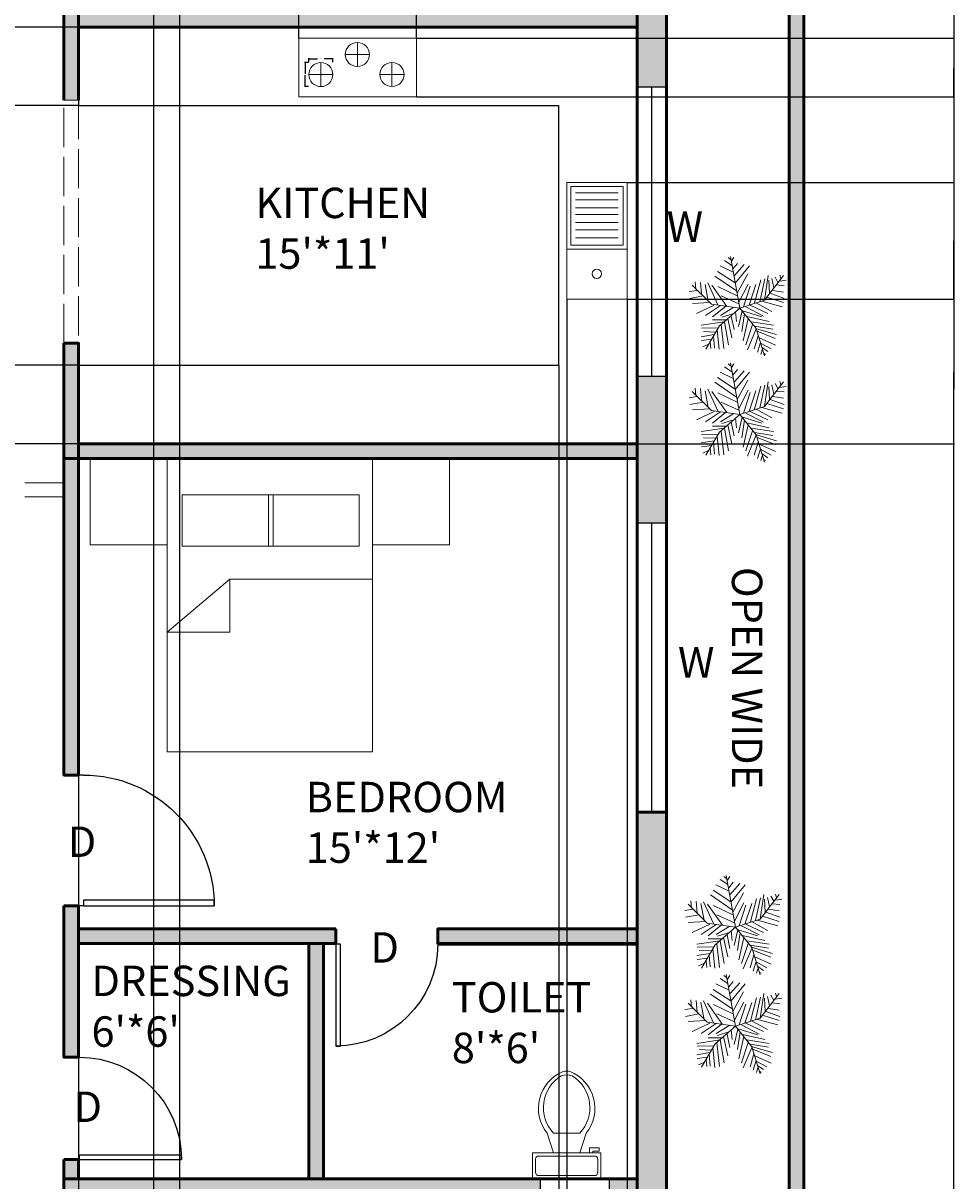
# Model space of a CAD drawing. Units: inches. Extents: x 2024 to 2594, y 643 to 1604.
# Tile 3 of 4: x 2309 to 2594, y 865 to 1219. Entities that reach past the tile are written whole.
import ezdxf

# ---------------------------------------------------------------- set-up
doc = ezdxf.new("R2010")
doc.units = ezdxf.units.IN
doc.linetypes.add('ACAD_ISO02W100', pattern=[15, 12, -3])
for name, color, linetype, lineweight in [('A-ANNO-DIMS', 2, 'Continuous', 18), ('A-ANNO-TEXT', 7, 'Continuous', 18), ('A-AREA-IDEN', 7, 'Continuous', 25), ('A-EQPM', 8, 'Continuous', 18), ('A-FLOR-CASE', 30, 'Continuous', 25), ('A-FLOR-FIXT', 8, 'Continuous', 18), ('A-WALL-OVHD', 50, 'ACAD_ISO02W100', 18), ('A-WALL-PATT', 50, 'Continuous', 13), ('C-PROP', 7, 'Continuous', 35), ('DOOR', 240, 'Continuous', 25), ('FUR', 212, 'Continuous', 18), ('TREE', 102, 'Continuous', 18), ('WALL', 50, 'Continuous', 50), ('WIN', 140, 'Continuous', 25)]:
    doc.layers.add(name, color=color, linetype=linetype, lineweight=lineweight)
doc.styles.get("Standard").update_dxf_attribs({"font": 'arial.ttf'})
doc.dimstyles.get("Standard").update_dxf_attribs({"dimtxt": 0.18, "dimasz": 0.18, "dimexe": 0.18, "dimexo": 0.0625, "dimgap": 0.09, "dimtad": 0, "dimtih": 1, "dimtoh": 1, "dimdec": 4, "dimzin": 0, "dimdsep": 46, "dimtxsty": 'Standard', "dimcen": 0.09, "dimadec": 0, "dimazin": 0, "dimtfac": 1, "dimtdec": 4, "dimtofl": 0, "dimtmove": 0, "dimatfit": 3, "dimfxl": 1, "dimtolj": 1, "dimtzin": 0, "dimarcsym": 0})

# ---------------------------------------------------------------- blocks, each defined once
blk = doc.blocks.new('*U4')
for p, q in [((9.5, -6), (9.5, -2)), ((-10, -8.5), (-8, -8.5)), ((-10, -9.5), (-10, -8.5)), ((-7, -9.5), (-10, -9.5)), ((-8, -8.5), (-8, -8)), ((-7, -8), (-7, -9.5)), ((-4, -8), (-6, -14)), ((4, -8), (6, -14)), ((4, -14), (-4, -14))]:
    blk.add_line(p, q)
blk.add_lwpolyline([(10.5, -8), (10.5, 0), (-10.5, 0), (-10.5, -8)], close=True)
for points in [[(-9.5, -2), (-9.5, -6)], [(8.5, -1), (-8.5, -1)], [(-8.5, -7), (8.5, -7)]]:
    blk.add_lwpolyline(points)
for centre, radius, start, end in [((-8.62, -1.88), 0.884, 81.8699, 188.1301), ((8.62, -1.88), 0.884, 351.8699, 98.1301), ((-8.62, -6.12), 0.884, 171.8699, 278.1301), ((8.62, -6.12), 0.884, 261.8699, 8.1301), ((3.52, -21.58), 12.17, 141.4691, 247.9714), ((4.2, -21.82), 11.33, 136.3677, 238.9468), ((-3.52, -21.58), 12.17, 292.0284, 38.5307), ((-4.2, -21.82), 11.33, 301.053, 43.6321), ((0, -27.88), 4, 245.7318, 294.2682), ((0, -29), 4, 254.8605, 285.1395)]:
    blk.add_arc(centre, radius, start, end)
blk = doc.blocks.new('*U2')
for p, q in [((0, 0), (0, -6)), ((40, 0), (40, -6))]:
    blk.add_line(p, q)
blk.add_lwpolyline([(0, 0), (0, 40), (1.75, 40), (1.75, 0)], close=True)
blk.add_arc((0, 0), 40, 0, 90)
blk = doc.blocks.new('*U6')
for p, q in [((-8.737, 47.138), (-17.069, 52.711)), ((-10.186, 53.64), (-13.084, 55.962)), ((0, 0), (-10.5, 57)), ((-9.099, 51.782), (-6.563, 55.962)), ((-5.114, 28.097), (-24.676, 40.636)), ((-7.288, 39.707), (-21.778, 46.673)), ((-7.65, 43.423), (-2.578, 49.46)), ((-5.839, 35.992), (4.667, 48.067)), ((-5.114, 27.632), (10.463, 46.673)), ((-48.585, 21.131), (-49.309, 29.026)), ((-43.513, 28.561), (-42.427, 15.558)), ((-38.442, 26.239), (-34.819, 7.663)), ((-35.544, 28.097), (-24.314, 3.947)), ((-3.665, 19.273), (-27.574, 35.527)), ((-2.941, 16.486), (8.652, 37.85)), ((-1.129, 6.734), (9.014, 26.704)), ((10.101, 3.483), (17.708, 26.239)), ((16.259, 5.805), (23.142, 31.348)), ((22.055, 7.198), (27.489, 32.277)), ((27, 9), (48, 36)), ((27.127, 9.056), (31.112, 35.992)), ((31.836, 30.883), (32.561, 16.486)), ((35.096, 32.741), (37.27, 22.524)), ((38.719, 34.134), (41.979, 28.561)), ((40.53, 25.775), (48.862, 24.846)), ((43.791, 29.954), (51.036, 30.883)), ((44.153, 36.456), (45.239, 32.741)), ((-47.498, 19.737), (-55.83, 18.344)), ((-40.615, 13.7), (-55.105, 10.913)), ((-31.5, 4.5), (-52.5, 25.5)), ((-14.533, 2.09), (-30.834, 25.31)), ((-24.314, 23.917), (-2.941, 13.7)), ((-20.691, 13.7), (-1.129, 4.876)), ((3.942, 1.625), (11.187, 24.381)), ((33.285, 16.486), (48.862, 10.913)), ((36.183, 19.737), (48.137, 17.88)), ((-33.37, 6.269), (-52.207, 5.34)), ((-28.299, 3.483), (-47.86, -5.805)), ((-21.416, 3.018), (-38.079, -8.128)), ((0, 0), (-31.5, 4.5)), ((-15.982, 2.09), (-30.11, -9.521)), ((0, 0), (-22.5, -19.5)), ((-6.563, 1.161), (-21.416, -8.128)), ((0, 0), (27, 9)), ((0, 0), (18, -22.5)), ((6.478, 1.625), (26.04, -8.592)), ((11.187, 3.483), (30.749, -5.805)), ((18.07, 5.805), (35.096, -3.483)), ((24.229, 7.663), (46.688, 1.625)), ((29.662, 12.307), (48.137, 6.269)), ((-6.563, -5.805), (-19.967, -9.985)), ((-13.446, -11.378), (-8.737, -32.741)), ((-9.461, -8.592), (-6.201, -23.453)), ((-4.752, -3.483), (-3.665, -14.629)), ((2.493, -3.019), (-1.491, -20.202)), ((1.769, -2.555), (24.229, -9.521)), ((5.029, -6.27), (2.131, -25.775)), ((9.014, -11.378), (3.58, -35.992)), ((7.565, -9.056), (32.198, -14.629)), ((-17.431, -15.094), (-42.789, -18.809)), ((-24.314, -21.596), (-42.427, -22.06)), ((-22.5, -19.5), (-37.5, -45)), ((-15.257, -12.772), (-30.11, -12.772)), ((-25.038, -23.918), (-22.865, -45.281)), ((-20.691, -18.345), (-17.793, -44.352)), ((-17.069, -15.094), (-12.721, -40.172)), ((14.085, -16.951), (6.478, -40.172)), ((18.07, -22.524), (8.289, -45.745)), ((12.274, -15.094), (36.907, -18.809)), ((16.259, -19.738), (36.183, -22.989)), ((18, -22.5), (27, -52.5)), ((18.433, -22.524), (40.53, -29.026)), ((19.157, -25.311), (38.719, -33.206)), ((-28.299, -29.026), (-42.789, -31.348)), ((-30.834, -34.135), (-42.427, -35.528)), ((-26.849, -26.24), (-40.253, -25.775)), ((-32.646, -36.921), (-31.921, -44.352)), ((-29.023, -30.884), (-27.936, -43.887)), ((20.244, -30.419), (15.897, -44.816)), ((22.78, -37.85), (19.519, -48.532)), ((21.331, -32.741), (39.081, -40.636)), ((-34.457, -39.708), (-40.978, -42.494)), ((22.78, -38.314), (34.372, -44.816)), ((24.591, -45.745), (23.142, -50.854)), ((24.591, -43.423), (30.749, -47.603)), ((26.764, -49.925), (28.213, -50.854))]:
    blk.add_line(p, q)
blk = doc.blocks.new('BED-DOUBLE-WITH-NIGHTSTANDS')
for p, q in [((36.91, 86.39), (36.91, 42.72)), ((36.91, 42.72), (53.2, 42.72)), ((53.2, 23.62), (36.91, 42.72)), ((53.2, 42.72), (53.2, 23.62))]:
    blk.add_line(p, q)
for points in [[(0, 86.39), (26.45, 86.39), (26.45, 110.01), (0, 110.01)], [(0, 23.62), (89.75, 23.62), (89.75, 86.39), (0, 86.39)], [(11.14, 54.55), (26.84, 54.55), (26.84, 82.37), (11.14, 82.37)], [(11.14, 28.22), (26.84, 28.22), (26.84, 56.03), (11.14, 56.03)], [(0, 0), (26.45, 0), (26.45, 23.62), (0, 23.62)]]:
    blk.add_lwpolyline(points, close=True)
blk = doc.blocks.new('COOKTOP-BURNER')
for p, q in [((3.69, 0), (3.69, 7.39)), ((0, 3.69), (7.39, 3.69))]:
    blk.add_line(p, q)
blk.add_circle((3.69, 3.69), 3.69)
blk = doc.blocks.new('WINDOW-EXTERIOR')
blk.add_line((4.5, 0), (4.5, 88.37))
blk.add_lwpolyline([(0, 0), (9, 0), (9, 88.37), (0, 88.37)], close=True)
blk = doc.blocks.new('*D21')
at = {"layer": 'A-ANNO-DIMS', "color": 0, "lineweight": -2, "transparency": 16777216}
for p, q in [((2396.73, 1207.18), (2396.73, 1208.4)), ((2396.91, 1208.22), (2399.4, 1208.22)), ((2403.94, 1208.22), (2401.44, 1208.22)), ((2404.12, 1207.18), (2404.12, 1208.4))]:
    blk.add_line(p, q, dxfattribs=at)
at = {"layer": 'A-ANNO-DIMS', "color": 0, "lineweight": 100, "transparency": 16777216}
for points in [[(2396.91, 1208.25), (2396.91, 1208.19), (2396.73, 1208.22)], [(2403.94, 1208.25), (2403.94, 1208.19), (2404.12, 1208.22)]]:
    blk.add_solid(points, dxfattribs=at)
at = {"layer": 'Defpoints', "color": 0, "lineweight": 100, "transparency": 16777216}
for p in [(2404.12, 1208.22), (2396.73, 1207.11), (2404.12, 1207.11)]:
    blk.add_point(p, dxfattribs=at)
at = {"layer": 'A-ANNO-DIMS', "color": 0, "transparency": 16777216, "insert": (2400.42, 1208.22), "char_height": 0.18, "attachment_point": 5}
blk.add_mtext('\\A1;BURNER 7 TYP.', dxfattribs=at)
blk = doc.blocks.new('*D22')
at = {"layer": 'A-ANNO-DIMS', "color": 0, "lineweight": -2, "transparency": 16777216}
for p, q in [((2396.67, 1207.11), (2395.44, 1207.11)), ((2395.62, 1206.93), (2395.62, 1203.6)), ((2395.62, 1199.91), (2395.62, 1203.24)), ((2396.67, 1199.73), (2395.44, 1199.73))]:
    blk.add_line(p, q, dxfattribs=at)
at = {"layer": 'A-ANNO-DIMS', "color": 0, "lineweight": 100, "transparency": 16777216}
for points in [[(2395.59, 1206.93), (2395.65, 1206.93), (2395.62, 1207.11)], [(2395.59, 1199.91), (2395.65, 1199.91), (2395.62, 1199.73)]]:
    blk.add_solid(points, dxfattribs=at)
at = {"layer": 'Defpoints', "color": 0, "lineweight": 100, "transparency": 16777216}
for p in [(2395.62, 1207.11), (2396.73, 1207.11), (2396.73, 1199.73)]:
    blk.add_point(p, dxfattribs=at)
at = {"layer": 'A-ANNO-DIMS', "color": 0, "transparency": 16777216, "insert": (2395.62, 1203.42), "char_height": 0.18, "attachment_point": 5}
blk.add_mtext('\\A1;7 TYP.', dxfattribs=at)
blk = doc.blocks.new('*D26')
at = {"layer": 'A-ANNO-DIMS', "color": 0, "lineweight": -2, "transparency": 16777216}
for p, q in [((2548.34, 1526.93), (2594.37, 1526.93)), ((2594.19, 1526.75), (2594.19, 1107.11)), ((2594.19, 687.11), (2594.19, 1106.75)), ((2548.34, 686.93), (2594.37, 686.93))]:
    blk.add_line(p, q, dxfattribs=at)
at = {"layer": 'A-ANNO-DIMS', "color": 0, "lineweight": 100, "transparency": 16777216}
for points in [[(2594.16, 1526.75), (2594.22, 1526.75), (2594.19, 1526.93)], [(2594.16, 687.11), (2594.22, 687.11), (2594.19, 686.93)]]:
    blk.add_solid(points, dxfattribs=at)
at = {"layer": 'Defpoints', "color": 0, "lineweight": 100, "transparency": 16777216}
for p in [(2548.27, 1526.93), (2594.19, 1526.93), (2548.27, 686.93)]:
    blk.add_point(p, dxfattribs=at)
at = {"layer": 'A-ANNO-DIMS', "color": 0, "transparency": 16777216, "insert": (2594.19, 1106.93), "char_height": 0.18, "attachment_point": 5}
blk.add_mtext('\\A1;840', dxfattribs=at)
blk = doc.blocks.new('*D37')
at = {"layer": 'A-ANNO-DIMS', "color": 0, "lineweight": -2, "transparency": 16777216}
for p, q in [((2326.27, 1217.99), (2326.27, 1603.82)), ((2326.45, 1603.64), (2359.59, 1603.64)), ((2393.52, 1603.64), (2360.38, 1603.64)), ((2393.7, 1214.56), (2393.7, 1603.82))]:
    blk.add_line(p, q, dxfattribs=at)
at = {"layer": 'A-ANNO-DIMS', "color": 0, "lineweight": 100, "transparency": 16777216}
for points in [[(2326.45, 1603.67), (2326.45, 1603.61), (2326.27, 1603.64)], [(2393.52, 1603.67), (2393.52, 1603.61), (2393.7, 1603.64)]]:
    blk.add_solid(points, dxfattribs=at)
at = {"layer": 'Defpoints', "color": 0, "lineweight": 100, "transparency": 16777216}
for p in [(2393.7, 1603.64), (2326.27, 1217.93), (2393.7, 1214.5)]:
    blk.add_point(p, dxfattribs=at)
at = {"layer": 'A-ANNO-DIMS', "color": 0, "transparency": 16777216, "insert": (2359.99, 1603.64), "char_height": 0.18, "attachment_point": 5}
blk.add_mtext('\\A1;67.43', dxfattribs=at)
blk = doc.blocks.new('*D38')
at = {"layer": 'A-ANNO-DIMS', "color": 0, "lineweight": -2, "transparency": 16777216}
for p, q in [((2393.7, 1214.56), (2393.7, 1603.82)), ((2393.88, 1603.64), (2411.26, 1603.64)), ((2429.57, 1603.64), (2412.19, 1603.64)), ((2429.75, 1214.56), (2429.75, 1603.82))]:
    blk.add_line(p, q, dxfattribs=at)
at = {"layer": 'A-ANNO-DIMS', "color": 0, "lineweight": 100, "transparency": 16777216}
for points in [[(2393.88, 1603.67), (2393.88, 1603.61), (2393.7, 1603.64)], [(2429.57, 1603.67), (2429.57, 1603.61), (2429.75, 1603.64)]]:
    blk.add_solid(points, dxfattribs=at)
at = {"layer": 'Defpoints', "color": 0, "lineweight": 100, "transparency": 16777216}
for p in [(2429.75, 1603.64), (2393.7, 1214.5), (2429.75, 1214.5)]:
    blk.add_point(p, dxfattribs=at)
at = {"layer": 'A-ANNO-DIMS', "color": 0, "transparency": 16777216, "insert": (2411.73, 1603.64), "char_height": 0.18, "attachment_point": 5}
blk.add_mtext('\\A1;36.046', dxfattribs=at)
blk = doc.blocks.new('*D39')
at = {"layer": 'A-ANNO-DIMS', "color": 0, "lineweight": -2, "transparency": 16777216}
for p, q in [((2429.81, 1214.5), (2594.37, 1214.5)), ((2594.19, 1214.32), (2594.19, 1205.74)), ((2594.19, 1196.8), (2594.19, 1205.38)), ((2429.81, 1196.62), (2594.37, 1196.62))]:
    blk.add_line(p, q, dxfattribs=at)
at = {"layer": 'A-ANNO-DIMS', "color": 0, "lineweight": 100, "transparency": 16777216}
for points in [[(2594.16, 1214.32), (2594.22, 1214.32), (2594.19, 1214.5)], [(2594.16, 1196.8), (2594.22, 1196.8), (2594.19, 1196.62)]]:
    blk.add_solid(points, dxfattribs=at)
at = {"layer": 'Defpoints', "color": 0, "lineweight": 100, "transparency": 16777216}
for p in [(2429.75, 1214.5), (2594.19, 1214.5), (2429.75, 1196.62)]:
    blk.add_point(p, dxfattribs=at)
at = {"layer": 'A-ANNO-DIMS', "color": 0, "transparency": 16777216, "insert": (2594.19, 1205.56), "char_height": 0.18, "attachment_point": 5}
blk.add_mtext('\\A1;17.88', dxfattribs=at)
blk = doc.blocks.new('*D40')
at = {"layer": 'A-ANNO-DIMS', "color": 0, "lineweight": -2, "transparency": 16777216}
for p, q in [((2326.27, 1114.37), (2326.27, 642.95)), ((2473.27, 1114.37), (2473.27, 642.95)), ((2326.45, 643.13), (2399.49, 643.13)), ((2473.09, 643.13), (2400.05, 643.13))]:
    blk.add_line(p, q, dxfattribs=at)
at = {"layer": 'A-ANNO-DIMS', "color": 0, "lineweight": 100, "transparency": 16777216}
for points in [[(2326.45, 643.16), (2326.45, 643.1), (2326.27, 643.13)], [(2473.09, 643.16), (2473.09, 643.1), (2473.27, 643.13)]]:
    blk.add_solid(points, dxfattribs=at)
at = {"layer": 'Defpoints', "color": 0, "lineweight": 100, "transparency": 16777216}
for p in [(2326.27, 1114.43), (2473.27, 1114.43), (2473.27, 643.13)]:
    blk.add_point(p, dxfattribs=at)
at = {"layer": 'A-ANNO-DIMS', "color": 0, "transparency": 16777216, "insert": (2399.77, 643.13), "char_height": 0.18, "attachment_point": 5}
blk.add_mtext('\\A1;147', dxfattribs=at)
blk = doc.blocks.new('*D41')
at = {"layer": 'A-ANNO-DIMS', "color": 0, "lineweight": -2, "transparency": 16777216}
for p, q in [((2473.27, 1114.37), (2473.27, 642.95)), ((2497.27, 1090.37), (2497.27, 642.95)), ((2473.45, 643.13), (2485.05, 643.13)), ((2497.09, 643.13), (2485.49, 643.13))]:
    blk.add_line(p, q, dxfattribs=at)
at = {"layer": 'A-ANNO-DIMS', "color": 0, "lineweight": 100, "transparency": 16777216}
for points in [[(2473.45, 643.16), (2473.45, 643.1), (2473.27, 643.13)], [(2497.09, 643.16), (2497.09, 643.1), (2497.27, 643.13)]]:
    blk.add_solid(points, dxfattribs=at)
at = {"layer": 'Defpoints', "color": 0, "lineweight": 100, "transparency": 16777216}
for p in [(2473.27, 1114.43), (2497.27, 1090.43), (2497.27, 643.13)]:
    blk.add_point(p, dxfattribs=at)
at = {"layer": 'A-ANNO-DIMS', "color": 0, "transparency": 16777216, "insert": (2485.27, 643.13), "char_height": 0.18, "attachment_point": 5}
blk.add_mtext('\\A1;24', dxfattribs=at)
blk = doc.blocks.new('*D42')
at = {"layer": 'A-ANNO-DIMS', "color": 0, "lineweight": -2, "transparency": 16777216}
for p, q in [((2326.21, 1114.43), (2024.29, 1114.43)), ((2024.47, 1114.25), (2024.47, 1102.61)), ((2024.47, 1090.61), (2024.47, 1102.25)), ((2326.21, 1090.43), (2024.29, 1090.43))]:
    blk.add_line(p, q, dxfattribs=at)
at = {"layer": 'A-ANNO-DIMS', "color": 0, "lineweight": 100, "transparency": 16777216}
for points in [[(2024.44, 1114.25), (2024.5, 1114.25), (2024.47, 1114.43)], [(2024.44, 1090.61), (2024.5, 1090.61), (2024.47, 1090.43)]]:
    blk.add_solid(points, dxfattribs=at)
at = {"layer": 'Defpoints', "color": 0, "lineweight": 100, "transparency": 16777216}
for p in [(2024.47, 1114.43), (2326.27, 1114.43), (2326.27, 1090.43)]:
    blk.add_point(p, dxfattribs=at)
at = {"layer": 'A-ANNO-DIMS', "color": 0, "transparency": 16777216, "insert": (2024.47, 1102.43), "char_height": 0.18, "attachment_point": 5}
blk.add_mtext('\\A1;24', dxfattribs=at)
blk = doc.blocks.new('*D43')
at = {"layer": 'A-ANNO-DIMS', "color": 0, "lineweight": -2, "transparency": 16777216}
for p, q in [((2326.21, 1193.93), (2024.29, 1193.93)), ((2024.47, 1193.75), (2024.47, 1154.36)), ((2024.47, 1114.61), (2024.47, 1154)), ((2326.21, 1114.43), (2024.29, 1114.43))]:
    blk.add_line(p, q, dxfattribs=at)
at = {"layer": 'A-ANNO-DIMS', "color": 0, "lineweight": 100, "transparency": 16777216}
for points in [[(2024.44, 1193.75), (2024.5, 1193.75), (2024.47, 1193.93)], [(2024.44, 1114.61), (2024.5, 1114.61), (2024.47, 1114.43)]]:
    blk.add_solid(points, dxfattribs=at)
at = {"layer": 'Defpoints', "color": 0, "lineweight": 100, "transparency": 16777216}
for p in [(2024.47, 1193.93), (2326.27, 1193.93), (2326.27, 1114.43)]:
    blk.add_point(p, dxfattribs=at)
at = {"layer": 'A-ANNO-DIMS', "color": 0, "transparency": 16777216, "insert": (2024.47, 1154.18), "char_height": 0.18, "attachment_point": 5}
blk.add_mtext('\\A1;79.5', dxfattribs=at)
blk = doc.blocks.new('*D44')
at = {"layer": 'A-ANNO-DIMS', "color": 0, "lineweight": -2, "transparency": 16777216}
for p, q in [((2326.21, 1217.93), (2024.29, 1217.93)), ((2024.47, 1217.75), (2024.47, 1206.11)), ((2024.47, 1194.11), (2024.47, 1205.75)), ((2326.21, 1193.93), (2024.29, 1193.93))]:
    blk.add_line(p, q, dxfattribs=at)
at = {"layer": 'A-ANNO-DIMS', "color": 0, "lineweight": 100, "transparency": 16777216}
for points in [[(2024.44, 1217.75), (2024.5, 1217.75), (2024.47, 1217.93)], [(2024.44, 1194.11), (2024.5, 1194.11), (2024.47, 1193.93)]]:
    blk.add_solid(points, dxfattribs=at)
at = {"layer": 'Defpoints', "color": 0, "lineweight": 100, "transparency": 16777216}
for p in [(2024.47, 1217.93), (2326.27, 1217.93), (2326.27, 1193.93)]:
    blk.add_point(p, dxfattribs=at)
at = {"layer": 'A-ANNO-DIMS', "color": 0, "transparency": 16777216, "insert": (2024.47, 1205.93), "char_height": 0.18, "attachment_point": 5}
blk.add_mtext('\\A1;24', dxfattribs=at)
blk = doc.blocks.new('*D45')
at = {"layer": 'A-ANNO-DIMS', "color": 0, "lineweight": -2, "transparency": 16777216}
for p, q in [((2494.21, 1134.64), (2594.37, 1134.64)), ((2594.19, 1134.46), (2594.19, 1112.71)), ((2594.19, 1090.61), (2594.19, 1112.35)), ((2497.34, 1090.43), (2594.37, 1090.43))]:
    blk.add_line(p, q, dxfattribs=at)
at = {"layer": 'A-ANNO-DIMS', "color": 0, "lineweight": 100, "transparency": 16777216}
for points in [[(2594.16, 1134.46), (2594.22, 1134.46), (2594.19, 1134.64)], [(2594.16, 1090.61), (2594.22, 1090.61), (2594.19, 1090.43)]]:
    blk.add_solid(points, dxfattribs=at)
at = {"layer": 'Defpoints', "color": 0, "lineweight": 100, "transparency": 16777216}
for p in [(2494.15, 1134.64), (2594.19, 1134.64), (2497.27, 1090.43)]:
    blk.add_point(p, dxfattribs=at)
at = {"layer": 'A-ANNO-DIMS', "color": 0, "transparency": 16777216, "insert": (2594.19, 1112.53), "char_height": 0.18, "attachment_point": 5}
blk.add_mtext('\\A1;44.21', dxfattribs=at)
blk = doc.blocks.new('*D46')
at = {"layer": 'A-ANNO-DIMS', "color": 0, "lineweight": -2, "transparency": 16777216}
for p, q in [((2494.21, 1170.35), (2594.37, 1170.35)), ((2594.19, 1170.17), (2594.19, 1152.67)), ((2594.19, 1134.82), (2594.19, 1152.31)), ((2494.21, 1134.64), (2594.37, 1134.64))]:
    blk.add_line(p, q, dxfattribs=at)
at = {"layer": 'A-ANNO-DIMS', "color": 0, "lineweight": 100, "transparency": 16777216}
for points in [[(2594.16, 1170.17), (2594.22, 1170.17), (2594.19, 1170.35)], [(2594.16, 1134.82), (2594.22, 1134.82), (2594.19, 1134.64)]]:
    blk.add_solid(points, dxfattribs=at)
at = {"layer": 'Defpoints', "color": 0, "lineweight": 100, "transparency": 16777216}
for p in [(2494.15, 1170.35), (2594.19, 1170.35), (2494.15, 1134.64)]:
    blk.add_point(p, dxfattribs=at)
at = {"layer": 'A-ANNO-DIMS', "color": 0, "transparency": 16777216, "insert": (2594.19, 1152.49), "char_height": 0.18, "attachment_point": 5}
blk.add_mtext('\\A1;35.71', dxfattribs=at)
blk = doc.blocks.new('*D47')
at = {"layer": 'A-ANNO-DIMS', "color": 0, "lineweight": -2, "transparency": 16777216}
for p, q in [((2475.68, 1134.57), (2475.68, 642.95)), ((2494.15, 1134.57), (2494.15, 642.95)), ((2475.86, 643.13), (2484.53, 643.13)), ((2493.97, 643.13), (2485.3, 643.13))]:
    blk.add_line(p, q, dxfattribs=at)
at = {"layer": 'A-ANNO-DIMS', "color": 0, "lineweight": 100, "transparency": 16777216}
for points in [[(2475.86, 643.16), (2475.86, 643.1), (2475.68, 643.13)], [(2493.97, 643.16), (2493.97, 643.1), (2494.15, 643.13)]]:
    blk.add_solid(points, dxfattribs=at)
at = {"layer": 'Defpoints', "color": 0, "lineweight": 100, "transparency": 16777216}
for p in [(2475.68, 1134.64), (2494.15, 1134.64), (2494.15, 643.13)]:
    blk.add_point(p, dxfattribs=at)
at = {"layer": 'A-ANNO-DIMS', "color": 0, "transparency": 16777216, "insert": (2484.91, 643.13), "char_height": 0.18, "attachment_point": 5}
blk.add_mtext('\\A1;18.47', dxfattribs=at)
blk = doc.blocks.new('*D48')
at = {"layer": 'A-ANNO-DIMS', "color": 0, "lineweight": -2, "transparency": 16777216}
for p, q in [((2249.77, 819.02), (2249.77, 1603.82)), ((2249.95, 1603.64), (2299.2, 1603.64)), ((2349.09, 1603.64), (2299.85, 1603.64)), ((2349.27, 860.99), (2349.27, 1603.82))]:
    blk.add_line(p, q, dxfattribs=at)
at = {"layer": 'A-ANNO-DIMS', "color": 0, "lineweight": 100, "transparency": 16777216}
for points in [[(2249.95, 1603.67), (2249.95, 1603.61), (2249.77, 1603.64)], [(2349.09, 1603.67), (2349.09, 1603.61), (2349.27, 1603.64)]]:
    blk.add_solid(points, dxfattribs=at)
at = {"layer": 'Defpoints', "color": 0, "lineweight": 100, "transparency": 16777216}
for p in [(2349.27, 1603.64), (2349.27, 860.93), (2249.77, 818.96)]:
    blk.add_point(p, dxfattribs=at)
at = {"layer": 'A-ANNO-DIMS', "color": 0, "transparency": 16777216, "insert": (2299.52, 1603.64), "char_height": 0.18, "attachment_point": 5}
blk.add_mtext('\\A1;99.5', dxfattribs=at)
blk = doc.blocks.new('*D51')
at = {"layer": 'A-ANNO-DIMS', "color": 0, "lineweight": -2, "transparency": 16777216}
for p, q in [((2349.27, 860.99), (2349.27, 1603.82)), ((2349.45, 1603.64), (2353.12, 1603.64)), ((2357.09, 1603.64), (2353.42, 1603.64)), ((2357.27, 860.99), (2357.27, 1603.82))]:
    blk.add_line(p, q, dxfattribs=at)
at = {"layer": 'A-ANNO-DIMS', "color": 0, "lineweight": 100, "transparency": 16777216}
for points in [[(2349.45, 1603.67), (2349.45, 1603.61), (2349.27, 1603.64)], [(2357.09, 1603.67), (2357.09, 1603.61), (2357.27, 1603.64)]]:
    blk.add_solid(points, dxfattribs=at)
at = {"layer": 'Defpoints', "color": 0, "lineweight": 100, "transparency": 16777216}
for p in [(2357.27, 1603.64), (2349.27, 860.93), (2357.27, 860.93)]:
    blk.add_point(p, dxfattribs=at)
at = {"layer": 'A-ANNO-DIMS', "color": 0, "transparency": 16777216, "insert": (2353.27, 1603.64), "char_height": 0.18, "attachment_point": 5}
blk.add_mtext('\\A1;8', dxfattribs=at)

msp = doc.modelspace()

# ---------------------------------------------------------------- hatches: boundary and pattern name
at = {"layer": 'A-WALL-PATT'}
h = msp.add_hatch(color=256, dxfattribs=at)
h.dxf.hatch_style = 1
h.paths.add_polyline_path([(2543.7727, 1526.9303), (2077.2727, 1526.9303), (2077.2727, 1522.4303), (2543.7727, 1522.4303)])
h.paths.add_polyline_path([(2077.2727, 1526.9303), (2068.2727, 1526.9303), (2068.2727, 1475.9303), (2077.2727, 1475.9303)])
h.paths.add_polyline_path([(2077.2727, 1475.9303), (2068.2727, 1475.9303), (2068.2727, 686.9303), (2077.2727, 686.9303)])
h.paths.add_polyline_path([(2548.2727, 1526.9303), (2543.7727, 1526.9303), (2543.7727, 1522.4303), (2543.7727, 691.4303), (2548.2727, 691.4303)])
h.paths.add_polyline_path([(2249.7727, 1078.4303), (2199.5227, 1078.4303), (2199.5227, 1073.9303), (2245.2727, 1073.9303), (2249.7727, 1073.9217)])
h.paths.add_polyline_path([(2249.7727, 1073.9217), (2245.2727, 1073.9217), (2245.2727, 935.5102), (2249.7727, 935.5102)])
h.paths.add_polyline_path([(2326.2727, 1121.201), (2321.7727, 1121.201), (2321.7727, 1085.9303), (2326.2727, 1085.9303), (2326.2727, 1090.4303)])
h.paths.add_polyline_path([(2497.2727, 1090.4303), (2326.2727, 1090.4303), (2326.2727, 1085.9303), (2497.2727, 1085.9303)])
h.paths.add_polyline_path([(2326.2727, 1085.9303), (2321.7727, 1085.9303), (2321.7727, 989.0099), (2326.2727, 989.0099)])
h.paths.add_polyline_path([(2199.1605, 1286.9303), (2077.2727, 1286.9303), (2077.2727, 1282.4303), (2199.1605, 1282.4303)])
h.paths.add_polyline_path([(2321.7727, 1286.9303), (2239.1605, 1286.9303), (2239.1605, 1282.4303), (2321.7727, 1282.4303)])
h.paths.add_polyline_path([(2245.2727, 881.9303), (2214.9534, 881.9303), (2214.9534, 877.4303), (2245.2727, 877.4303)])
h.paths.add_polyline_path([(2118.9166, 881.9303), (2077.2727, 881.9303), (2077.2727, 877.4303), (2118.9166, 877.4303)])
h.paths.add_polyline_path([(2249.7727, 889.4074), (2246.315, 889.4074), (2245.2727, 889.4074), (2245.2727, 872.2078), (2249.7727, 872.2078)])
h.paths.add_polyline_path([(2405.0472, 941.9303), (2326.2727, 941.9303), (2326.2727, 937.4303), (2405.0472, 937.4303)])
h.paths.add_polyline_path([(2326.2727, 949.0099), (2321.7727, 949.0099), (2321.7727, 902.6727), (2326.2727, 902.6727)])
h.paths.add_polyline_path([(2326.2727, 871.366), (2321.7727, 871.366), (2321.7727, 865.4303), (2326.2727, 865.4303)])
h.paths.add_polyline_path([(2401.2727, 937.4303), (2396.7727, 937.4303), (2396.7727, 865.4303), (2401.2727, 865.4303)])
h.paths.add_polyline_path([(2497.2727, 941.9303), (2436.2168, 941.9303), (2436.2168, 937.4303), (2497.2727, 937.4303)])
h.paths.add_polyline_path([(2506.2727, 977.6959), (2497.2727, 977.6959), (2497.2727, 745.6665), (2506.2727, 745.6665)])
h.paths.add_polyline_path([(2497.2727, 754.6665), (2309.6667, 754.6665), (2309.6667, 745.6665), (2497.2727, 745.6665)])
h.paths.add_polyline_path([(2258.2092, 754.6665), (2245.2727, 754.6665), (2245.2727, 745.6665), (2258.2092, 745.6665)])
h.paths.add_polyline_path([(2249.7727, 772.853), (2248.7304, 772.853), (2245.2727, 772.853), (2245.2727, 754.6665), (2249.7727, 754.6665)])
h.paths.add_polyline_path([(2249.7727, 825.5234), (2245.2727, 825.5234), (2245.2727, 818.9558), (2248.7304, 818.9558), (2249.7727, 818.9558)])
h.paths.add_polyline_path([(2105.513, 1078.4303), (2077.2727, 1078.4303), (2077.2727, 1073.9303), (2105.513, 1073.9303)])
h.paths.add_polyline_path([(2326.2727, 1466.9303), (2321.7727, 1466.9303), (2321.7727, 1267.3126), (2326.2727, 1267.3126)])
h.paths.add_polyline_path([(2405.7727, 1466.9303), (2401.2727, 1466.9303), (2401.2727, 1438.953), (2405.7727, 1438.953)])
h.paths.add_polyline_path([(2405.7727, 1398.953), (2401.2727, 1398.953), (2401.2727, 1394.9303), (2405.7727, 1394.9303)])
h.paths.add_polyline_path([(2467.5339, 860.9303), (2467.5339, 865.4303), (2321.7727, 865.4303), (2321.7727, 860.9303)])
h.paths.add_polyline_path([(2488.7331, 865.4303), (2488.7331, 860.9303), (2497.2727, 860.9303), (2497.2727, 865.4303)])
h = msp.add_hatch(color=256, dxfattribs=at)
h.dxf.hatch_style = 1
h.paths.add_polyline_path([(2257.2361, 1475.9303), (2200.6585, 1475.9303), (2200.6585, 1466.9303), (2257.2361, 1466.9303)])
h.paths.add_polyline_path([(2112.2929, 1475.9303), (2077.2727, 1475.9303), (2077.2727, 1466.9303), (2112.2929, 1466.9303)])
h.paths.add_polyline_path([(2420.3831, 1475.9303), (2297.506, 1475.9303), (2297.506, 1466.9303), (2321.7727, 1466.9303), (2420.3831, 1466.9303)])
h.paths.add_polyline_path([(2249.7727, 1466.9303), (2245.2727, 1466.9303), (2245.2727, 1366.4303), (2249.7727, 1366.4303)])
h.paths.add_polyline_path([(2253.6326, 1370.9303), (2249.7727, 1370.9303), (2249.7727, 1366.4303), (2253.6326, 1366.4303)])
h.paths.add_polyline_path([(2321.7727, 1370.9303), (2293.6326, 1370.9303), (2293.6326, 1366.4303), (2321.7727, 1366.4303)])
h.paths.add_polyline_path([(2333.369, 1394.9303), (2326.2727, 1394.9303), (2326.2727, 1390.4303), (2333.369, 1390.4303)])
h.paths.add_polyline_path([(2506.2727, 1475.9303), (2460.6529, 1475.9303), (2460.6529, 1466.9303), (2474.0052, 1466.9303), (2497.2727, 1466.9303), (2497.2727, 1357.1459), (2506.2727, 1357.1459)])
h.paths.add_polyline_path([(2497.2727, 1394.9303), (2378.1903, 1394.9303), (2378.1903, 1390.4303), (2497.2727, 1390.4303)])
h.paths.add_polyline_path([(2506.2727, 1268.7803), (2497.2727, 1268.7803), (2497.2727, 1222.4303), (2497.2727, 1199.5194), (2506.2727, 1199.5194)])
h.paths.add_polyline_path([(2497.2727, 1222.4303), (2326.2727, 1222.4303), (2326.2727, 1217.9303), (2497.2727, 1217.9303)])
h.paths.add_polyline_path([(2326.2727, 1217.9303), (2326.2727, 1227.3126), (2321.7727, 1227.3126), (2321.7727, 1195.5957), (2326.2727, 1195.5957)])
h.paths.add_polyline_path([(2506.2727, 1111.1538), (2497.2727, 1111.1538), (2497.2727, 1085.9303), (2497.2727, 1066.0615), (2506.2727, 1066.0615)])

# ---------------------------------------------------------------- linework, layer by layer
at = {"layer": 'A-EQPM'}
msp.add_lwpolyline([(2393.7024, 1214.5024), (2429.7486, 1214.5024), (2429.7486, 1196.6208), (2393.7024, 1196.6208)], close=True, dxfattribs=at)
at = {"layer": 'A-FLOR-CASE'}
for p, q in [((2326.2727, 1217.9303), (2326.2727, 1193.9303)), ((2326.2727, 1193.9303), (2473.2727, 1193.9303)), ((2473.2727, 1114.4303), (2473.2727, 1193.9303)), ((2326.2727, 1090.4303), (2326.2727, 1114.4303)), ((2326.2727, 1114.4303), (2473.2727, 1114.4303))]:
    msp.add_line(p, q, dxfattribs=at)
at = {"layer": 'A-FLOR-FIXT'}
for p, q in [((2478.3758, 1167.1839), (2491.4331, 1167.1839)), ((2478.3758, 1165.0522), (2491.4331, 1165.0522)), ((2478.3758, 1162.6646), (2491.4331, 1162.6646)), ((2478.3758, 1160.5329), (2491.4331, 1160.5329)), ((2478.3758, 1158.1454), (2491.4331, 1158.1454)), ((2478.3758, 1155.8431), (2491.4331, 1155.8431)), ((2478.3758, 1153.4556), (2491.4331, 1153.4556)), ((2475.6764, 1149.9596), (2494.1482, 1149.9596))]:
    msp.add_line(p, q, dxfattribs=at)
for points in [[(2475.6764, 1170.348), (2494.1482, 1170.348), (2494.1482, 1134.6374), (2475.6764, 1134.6374)], [(2476.9249, 1151.1533), (2492.9693, 1151.1533), (2492.9693, 1169.1451), (2476.9249, 1169.1451)]]:
    msp.add_lwpolyline(points, close=True, dxfattribs=at)
msp.add_circle((2484.9123, 1142.4559), 1.4205, dxfattribs=at)
at = {"layer": 'A-WALL-OVHD'}
for p, q in [((2321.7727, 1195.5957), (2326.2727, 1195.5957)), ((2321.7727, 1121.201), (2326.2727, 1121.201))]:
    msp.add_line(p, q, dxfattribs=at)
for points in [[(2321.7727, 1195.5957), (2326.2727, 1195.5957), (2326.2727, 1121.201), (2321.7727, 1121.201)], [(2249.7727, 1078.4303), (2321.7727, 1078.4303), (2321.7727, 1074.2238), (2249.7727, 1074.2238)]]:
    msp.add_lwpolyline(points, close=True, dxfattribs=at)
at = {"layer": 'C-PROP'}
msp.add_line((2548.2727, 1526.9303), (2548.2727, 686.9303), dxfattribs=at)
msp.add_lwpolyline([(2548.2727, 686.9303), (2068.2727, 686.9303), (2068.2727, 1526.9303), (2548.2727, 1526.9303)], close=True, dxfattribs=at)
at = {"layer": 'WALL'}
for p, q in [((2506.2727, 1475.9303), (2506.2727, 745.6665)), ((2497.2727, 1466.9303), (2497.2727, 754.6665)), ((2321.7727, 1227.3126), (2321.7727, 1195.5957)), ((2326.2727, 1227.3126), (2326.2727, 1195.5957)), ((2497.2727, 1217.9303), (2326.2727, 1217.9303)), ((2497.2727, 1217.9303), (2497.2727, 1085.9303)), ((2321.7727, 1121.201), (2321.7727, 1085.9303)), ((2326.2727, 1121.201), (2326.2727, 1090.4303)), ((2321.7727, 989.0099), (2321.7727, 1090.4303)), ((2497.2727, 1090.4303), (2326.2727, 1090.4303)), ((2497.2727, 1085.9303), (2326.2727, 1085.9303)), ((2326.2727, 989.0099), (2326.2727, 1085.9303)), ((2497.2727, 1085.9303), (2497.2727, 941.9303)), ((2321.7727, 902.6727), (2321.7727, 949.0099)), ((2326.2727, 941.9303), (2326.2727, 949.0099)), ((2405.0472, 941.9303), (2326.2727, 941.9303)), ((2497.2727, 941.9303), (2436.2168, 941.9303)), ((2396.7727, 937.4303), (2326.2727, 937.4303)), ((2326.2727, 902.6727), (2326.2727, 937.4303)), ((2396.7727, 865.4303), (2396.7727, 937.4303)), ((2401.2727, 865.4303), (2401.2727, 937.4303)), ((2405.0472, 937.4303), (2401.2727, 937.4303)), ((2497.2727, 937.4303), (2436.2168, 937.4303)), ((2497.2727, 937.4303), (2497.2727, 865.4303)), ((2321.7727, 860.9303), (2321.7727, 871.366)), ((2326.2727, 865.4303), (2326.2727, 871.366)), ((2396.7727, 865.4303), (2326.2727, 865.4303)), ((2497.2727, 865.4303), (2401.2727, 865.4303))]:
    msp.add_line(p, q, dxfattribs=at)
for points in [[(2543.7727, 691.4303), (2548.2727, 691.4303), (2548.2727, 1526.9303), (2543.7727, 1526.9303)], [(2321.7727, 1121.201), (2326.2727, 1121.201), (2326.2727, 1085.9303), (2321.7727, 1085.9303)], [(2326.2727, 1085.9303), (2497.2727, 1085.9303), (2497.2727, 1090.4303), (2326.2727, 1090.4303)], [(2321.7727, 1085.9303), (2326.2727, 1085.9303), (2326.2727, 989.0099), (2321.7727, 989.0099)], [(2497.2727, 977.6959), (2506.2727, 977.6959), (2506.2727, 745.6665), (2497.2727, 745.6665)], [(2321.7727, 949.0099), (2326.2727, 949.0099), (2326.2727, 902.6727), (2321.7727, 902.6727)], [(2405.0472, 941.9303), (2326.2727, 941.9303), (2326.2727, 937.4303), (2405.0472, 937.4303)], [(2436.2168, 937.2549), (2497.2727, 937.2549), (2497.2727, 941.9303), (2436.2168, 941.9303)], [(2396.7727, 937.4303), (2401.2727, 937.4303), (2401.2727, 865.4303), (2396.7727, 865.4303)], [(2321.7727, 871.366), (2326.2727, 871.366), (2326.2727, 865.4303), (2321.7727, 865.4303)], [(2321.7727, 865.4303), (2497.2727, 865.4303), (2497.2727, 860.9303), (2321.7727, 860.9303)]]:
    msp.add_lwpolyline(points, close=True, dxfattribs=at)
msp.add_lwpolyline([(2077.2727, 1522.4303), (2543.7727, 1522.4303), (2543.7727, 691.4303), (2258.7401, 691.4303)], dxfattribs=at)
at = {"layer": 'WIN'}
msp.add_lwpolyline([(2467.5339, 860.9303), (2488.7331, 860.9303), (2488.7331, 865.4303), (2467.5339, 865.4303)], close=True, dxfattribs=at)

# ---------------------------------------------------------------- block references
at = {"layer": 'A-EQPM', "rotation": 180}
for p in [(2415.2938, 1213.2431), (2425.8808, 1207.1147)]:
    msp.add_blockref('COOKTOP-BURNER', p, dxfattribs=at)
at = {"layer": 'A-EQPM'}
msp.add_blockref('COOKTOP-BURNER', (2396.73, 1199.727), dxfattribs=at)
at = {"layer": 'A-FLOR-FIXT', "rotation": 180}
msp.add_blockref('*U4', (2475.6622, 865.4303), dxfattribs=at)
at = {"layer": 'DOOR', "xscale": -1, "rotation": 270}
msp.add_blockref('*U2', (2327.7727, 949.0099), dxfattribs=at)
at = {"layer": 'DOOR'}
for p, xscale, yscale, zscale, rotation in [((2405.0472, 937.2549), -0.7792407489926956, 0.7792407489926956, 0.7792407489926956, 180), ((2326.4687, 871.366), -0.7826684444065343, 0.7826684444065343, 0.7826684444065343, 270)]:
    msp.add_blockref('*U2', p, dxfattribs=dict(at, xscale=xscale, yscale=yscale, zscale=zscale, rotation=rotation))
at = {"layer": 'FUR', "rotation": 270.0000000000002}
msp.add_blockref('BED-DOUBLE-WITH-NIGHTSTANDS', (2329.8008, 1085.9307), dxfattribs=at)
at = {"layer": 'TREE', "xscale": 0.2775790715638129, "yscale": 0.2775790715638129, "zscale": 0.2775790715638129}
for p in [(2528.6995, 1131.8904), (2528.6995, 1099.3696), (2527.3899, 942.4651), (2527.3899, 912.1356)]:
    msp.add_blockref('*U6', p, dxfattribs=at)
at = {"layer": 'WIN'}
for p in [(2497.273, 1111.1539), (2497.273, 977.696)]:
    msp.add_blockref('WINDOW-EXTERIOR', p, dxfattribs=at)

# ---------------------------------------------------------------- texts
at = {"layer": 'A-ANNO-TEXT', "char_height": 9.3008, "attachment_point": 1}
for s, insert in [('W', (2506.2727, 1161.5035)), ('W', (2509.7538, 1028.1686)), ('D', (2322.9468, 973.2611)), ('D', (2415.6167, 940.9199)), ('D', (2324.7127, 892.152))]:
    msp.add_mtext_dynamic_manual_height_columns(s, width=384.915388, gutter_width=46.5039, heights=[0], dxfattribs=dict(at, insert=insert))
at = {"layer": 'A-AREA-IDEN', "char_height": 9.30079, "attachment_point": 1}
for s, insert in [("KITCHEN\\P15'*11'", (2380.3985, 1168.7747)), ("BEDROOM\\P15'*12'", (2395.8164, 986.9518)), ("DRESSING\\P6'*6'", (2330.2159, 930.6838)), ("TOILET\\P8'*6'", (2440.5248, 925.667))]:
    msp.add_mtext_dynamic_manual_height_columns(s, width=384.915388, gutter_width=46.5039, heights=[0], dxfattribs=dict(at, insert=insert))
at = {"layer": 'A-AREA-IDEN', "insert": (2535.5609, 1052.731), "char_height": 9.30079, "attachment_point": 1, "rotation": 270}
msp.add_mtext_dynamic_manual_height_columns('OPEN WIDE', width=384.915388, gutter_width=46.5039, heights=[0], dxfattribs=at)

# ---------------------------------------------------------------- dimensions: what is measured, and where the dimension line sits
at = {"layer": 'A-ANNO-DIMS'}
for base, p1, p2, override, picture, middle in [((2349.2727, 1603.6424), (2249.7727, 818.9558), (2349.2727, 860.9303), {"dimdec": 1, "dimlfac": 1, "dimrnd": 0, "dimzin": 0, "dimdsep": 46, "dimlunit": 2}, '*D48', (2299.5227, 1603.6424)), ((2393.7024, 1603.6424), (2326.2727, 1217.9303), (2393.7024, 1214.5024), {"dimdec": 2, "dimlfac": 1, "dimrnd": 0, "dimzin": 0, "dimdsep": 46, "dimlunit": 2}, '*D37', (2359.9876, 1603.6424)), ((2357.2727, 1603.6424), (2349.2727, 860.9303), (2357.2727, 860.9303), {"dimdec": 0, "dimlfac": 1, "dimrnd": 0, "dimzin": 0, "dimdsep": 46, "dimlunit": 2}, '*D51', (2353.2727, 1603.6424)), ((2429.7486, 1603.6424), (2393.7024, 1214.5024), (2429.7486, 1214.5024), {"dimdec": 3, "dimlfac": 1, "dimrnd": 0, "dimzin": 0, "dimdsep": 46, "dimlunit": 2}, '*D38', (2411.7255, 1603.6424)), ((2494.1482, 643.1303), (2475.6764, 1134.6374), (2494.1482, 1134.6374), {"dimdec": 2, "dimlfac": 1, "dimrnd": 0, "dimzin": 0, "dimdsep": 46, "dimlunit": 2}, '*D47', (2484.9123, 643.1303)), ((2473.2727, 643.1303), (2326.2727, 1114.4303), (2473.2727, 1114.4303), {"dimdec": 0, "dimlfac": 1, "dimrnd": 0, "dimzin": 0, "dimdsep": 46, "dimlunit": 2}, '*D40', (2399.7727, 643.1303)), ((2497.2727, 643.1303), (2473.2727, 1114.4303), (2497.2727, 1090.4303), {"dimdec": 0, "dimlfac": 1, "dimrnd": 0, "dimzin": 0, "dimdsep": 46, "dimlunit": 2}, '*D41', (2485.2727, 643.1303))]:
    dim = msp.add_linear_dim(base=base, p1=p1, p2=p2, dimstyle='Standard', override=override, dxfattribs=at)
    dim.commit()
    dim.dimension.update_dxf_attribs({"geometry": picture, "text_midpoint": middle})
for base, p1, p2, override, picture, middle in [((2594.1903, 1526.9303), (2548.2727, 686.9303), (2548.2727, 1526.9303), {"dimdec": 0, "dimlfac": 1, "dimrnd": 0, "dimzin": 0, "dimdsep": 46, "dimlunit": 2}, '*D26', (2594.1903, 1106.9303)), ((2024.4727, 1217.9303), (2326.2727, 1193.9303), (2326.2727, 1217.9303), {"dimdec": 0, "dimlfac": 1, "dimrnd": 0, "dimzin": 0, "dimdsep": 46, "dimlunit": 2}, '*D44', (2024.4727, 1205.9303)), ((2594.1903, 1214.5024), (2429.7486, 1196.6208), (2429.7486, 1214.5024), {"dimdec": 2, "dimlfac": 1, "dimrnd": 0, "dimzin": 0, "dimdsep": 46, "dimlunit": 2}, '*D39', (2594.1903, 1205.5616)), ((2024.4727, 1193.9303), (2326.2727, 1114.4303), (2326.2727, 1193.9303), {"dimdec": 1, "dimlfac": 1, "dimrnd": 0, "dimzin": 0, "dimdsep": 46, "dimlunit": 2}, '*D43', (2024.4727, 1154.1803)), ((2594.1903, 1170.348), (2494.1482, 1134.6374), (2494.1482, 1170.348), {"dimdec": 2, "dimlfac": 1, "dimrnd": 0, "dimzin": 0, "dimdsep": 46, "dimlunit": 2}, '*D46', (2594.1903, 1152.4927)), ((2594.1903, 1134.6374), (2497.2727, 1090.4303), (2494.1482, 1134.6374), {"dimdec": 2, "dimlfac": 1, "dimrnd": 0, "dimzin": 0, "dimdsep": 46, "dimlunit": 2}, '*D45', (2594.1903, 1112.5339)), ((2024.4727, 1114.4303), (2326.2727, 1090.4303), (2326.2727, 1114.4303), {"dimdec": 0, "dimlfac": 1, "dimrnd": 0, "dimzin": 0, "dimdsep": 46, "dimlunit": 2}, '*D42', (2024.4727, 1102.4303))]:
    dim = msp.add_linear_dim(base=base, p1=p1, p2=p2, angle=90, dimstyle='Standard', override=override, dxfattribs=at)
    dim.commit()
    dim.dimension.update_dxf_attribs({"geometry": picture, "text_midpoint": middle})
dim = msp.add_linear_dim(base=(2404.1182, 1208.2229), p1=(2396.7305, 1207.1147), p2=(2404.1182, 1207.1147), text='BURNER <> TYP.', dimstyle='Standard', override={"dimdec": 0, "dimlfac": 1, "dimrnd": 0, "dimzin": 0, "dimdsep": 46, "dimlunit": 2}, dxfattribs=at)
dim.commit()
dim.dimension.update_dxf_attribs({"geometry": '*D21', "text_midpoint": (2400.4243, 1208.2229)})
dim = msp.add_linear_dim(base=(2395.6223, 1207.1147), p1=(2396.7305, 1199.727), p2=(2396.7305, 1207.1147), angle=90, text='<> TYP.', dimstyle='Standard', override={"dimdec": 0, "dimlfac": 1, "dimrnd": 0, "dimzin": 0, "dimdsep": 46, "dimlunit": 2}, dxfattribs=at)
dim.commit()
dim.dimension.update_dxf_attribs({"geometry": '*D22', "text_midpoint": (2395.6223, 1203.4208)})

doc.saveas('drawing.dxf')
